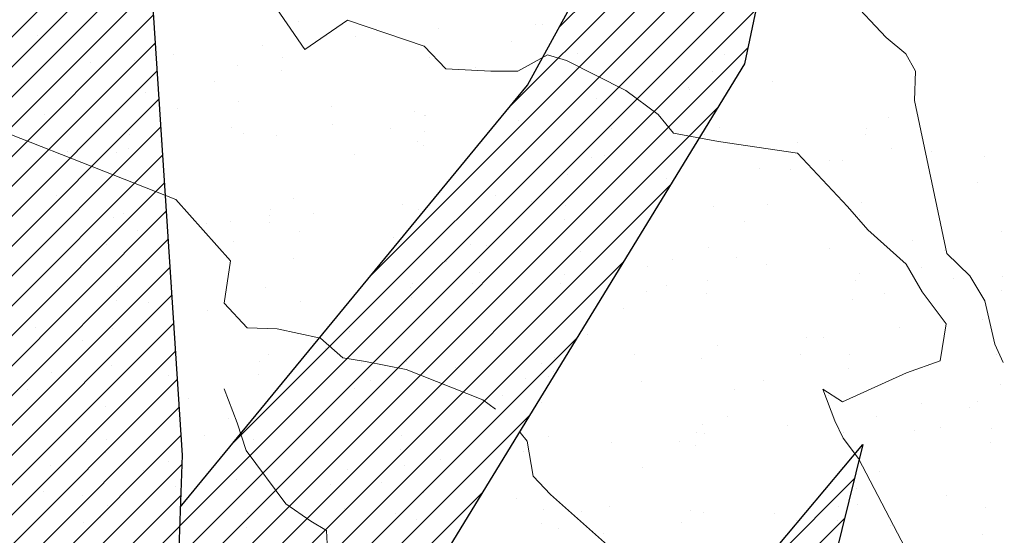
# Model space of a CAD drawing. Units: inches. Extents: x 1986 to 21484, y -1816 to 2016.
# Tile 74 of 85: x 3669.485 to 3676.656, y 1894.917 to 1898.672. Entities that reach past the tile are written whole.
import ezdxf

# ---------------------------------------------------------------- set-up
doc = ezdxf.new("R2010")
doc.units = ezdxf.units.IN
doc.layers.add('L-PLNT', color=84, linetype='Continuous', lineweight=13)
doc.layers.add('vfolhas', color=114, linetype='Continuous', lineweight=5)
doc.layers.add('vfolha2', color=110, linetype='Continuous')
doc.layers.add('vfolhas2', color=102, linetype='Continuous')
pattern_1 = [(45, (-2446.5133113, 50.986076), (-0.004419417382, 0.004419417382), [])]

# ---------------------------------------------------------------- blocks, each defined once
blk = doc.blocks.new('arbusto_PB_verde_grande')
at = {"layer": 'vfolha2'}
h = blk.add_hatch(dxfattribs=at)
h.set_pattern_fill('ANSI31', color=256, scale=0.05, style=0)
h.set_pattern_definition(pattern_1)
h.paths.add_polyline_path([(0.02944, 0.35651), (0.00028, 0.09048), (0.02625, -0.03934), (0.047, 0.06233), (0.06189, 0.09731), (0.09372, 0.26573), (0.09955, 0.43473), (0.08789, 0.61313), (0.0645, 0.72266), (0.04988, 0.6851), (0.0236, 0.51294)])
h.paths.add_polyline_path([(0.30106, 0.43789), (0.14225, 0.24871), (0.26685, 0.30022)])
h.paths.add_polyline_path([(0.37995, 0.22817), (0.23697, 0.15193), (0.18428, 0.09364), (0.11122, 0.04358), (0.02625, -0.03934), (0.28061, 0.04667), (0.36829, 0.07798), (0.46756, 0.11239), (0.61068, 0.19376), (0.71585, 0.27823), (0.55813, 0.25948)])
h.paths.add_polyline_path([(0.56101, -0.29441), (0.72752, -0.32573), (0.59024, -0.2412), (0.42962, -0.15982), (0.02625, -0.03934), (0.14922, -0.14107), (0.18838, -0.16604), (0.41501, -0.24435)])
h.paths.add_polyline_path([(-0.27429, -0.44776), (-0.30352, -0.72628), (-0.23923, -0.64175), (-0.15457, -0.45716), (0.02625, -0.03934), (-0.16328, -0.25376)])
h.paths.add_polyline_path([(-0.51963, -0.24744), (-0.67736, -0.32573), (-0.59558, -0.35072), (-0.40574, -0.32882), (-0.21007, -0.20995), (0.02625, -0.03934), (-0.14874, -0.06595), (-0.31518, -0.09101), (-0.41452, -0.15048)])
h.paths.add_polyline_path([(-0.52546, 0.25007), (-0.70947, 0.24698), (-0.51963, 0.1093), (-0.32979, 0.02167), (-0.07567, -0.0128), (-0.04234, -0.02148), (-0.35024, 0.1312)])
at = {"layer": 'vfolhas'}
h = blk.add_hatch(dxfattribs=at)
h.set_pattern_fill('ANSI31', color=256, scale=0.05, style=0)
h.set_pattern_definition(pattern_1)
h.paths.add_polyline_path([(-0.07279, 0.50669), (-0.18085, 0.65063), (-0.2334, 0.67253), (-0.20712, 0.53176), (-0.10785, 0.25007), (0.02625, -0.03934), (0.00028, 0.09048), (0.00816, 0.16241), (-0.04939, 0.29079)])
h.paths.add_polyline_path([(0.09902, 0.41929), (0.09372, 0.26573), (0.07906, 0.18814), (0.15506, 0.36901), (0.26606, 0.5505), (0.28356, 0.63504), (0.2485, 0.68819), (0.25145, 0.63504), (0.20178, 0.54426)])
h.paths.add_polyline_path([(0.12295, 0.24073), (0.047, 0.06233), (0.02625, -0.03934), (0.11122, 0.04358), (0.18428, 0.09364), (0.27478, 0.19376), (0.3215, 0.25323), (0.44129, 0.38467), (0.47634, 0.57866), (0.41789, 0.45347), (0.28939, 0.30954)])
h.paths.add_polyline_path([(0.58145, -0.03779), (0.70707, 0.01536), (0.78591, 0.04667), (0.74796, 0.06549), (0.62818, 0.08423), (0.52595, 0.09048), (0.39745, 0.04358), (0.02625, -0.03934), (0.25728, -0.03154), (0.43834, -0.0347)])
h.paths.add_polyline_path([(0.52022, -0.03647), (0.43834, -0.0347), (0.25728, -0.03154), (0.02625, -0.03934), (0.17964, -0.08515), (0.53768, -0.13167), (0.69541, -0.15357), (0.78591, -0.07852), (0.70413, -0.10042)])
h.paths.add_polyline_path([(0.27189, -0.21929), (0.14922, -0.14107), (0.02625, -0.03934), (0.15794, -0.31007), (0.29522, -0.42585), (0.41789, -0.49157), (0.56396, -0.56669), (0.5114, -0.48532), (0.39456, -0.34139)])
h.paths.add_polyline_path([(-0.05818, -0.47591), (-0.02312, -0.61984), (0.047, -0.80134), (0.08494, -0.59794), (0.07911, -0.4071), (0.03527, -0.25376), (0.02625, -0.03934), (-0.03773, -0.26001)])
h.paths.add_polyline_path([(-0.24218, 0.14054), (-0.11073, 0.06858), (0.02625, -0.03934), (-0.04235, 0.10871), (-0.21007, 0.23757), (-0.36485, 0.33145), (-0.47874, 0.40341), (-0.54303, 0.46288), (-0.49041, 0.33145), (-0.39408, 0.22192)])
at = {"layer": 'vfolha2'}
for p, q in [((0.08789, 0.61313), (0.09955, 0.43473)), ((0.14339, 0.25007), (0.30106, 0.43789)), ((0.30106, 0.43789), (0.26606, 0.29704)), ((0.09955, 0.43473), (0.09372, 0.26573))]:
    blk.add_line(p, q, dxfattribs=at)
at = {"layer": 'vfolhas2'}
for p, q in [((0.20178, 0.54426), (0.25145, 0.63504)), ((0.28356, 0.63504), (0.26606, 0.5505)), ((0.26606, 0.5505), (0.15506, 0.36901)), ((0.09902, 0.41929), (0.20178, 0.54426))]:
    blk.add_line(p, q, dxfattribs=at)
blk = doc.blocks.new('PLANT-SHRUB')
for p, q in [((2150.9894, 1887.1078), (2150.9894, 1887.1078)), ((2150.8411, 1886.9754), (2150.8411, 1886.9754)), ((2151.2728, 1886.0864), (2151.4706, 1886.7919)), ((2150.994, 1886.7216), (2150.994, 1886.7216)), ((2150.4934, 1886.6568), (2150.4934, 1886.6568)), ((2150.4197, 1886.5893), (2150.4197, 1886.5893)), ((2151.4419, 1886.6009), (2151.4419, 1886.6009)), ((2150.1488, 1886.3993), (2150.1488, 1886.3993)), ((2150.3568, 1886.3719), (2150.3568, 1886.3719)), ((2150.4298, 1886.3651), (2150.4298, 1886.3651)), ((2150.0259, 1886.2961), (2149.9795, 1886.157)), ((2150.6817, 1886.3292), (2150.6817, 1886.3292)), ((2151.5093, 1886.3263), (2151.5093, 1886.3263)), ((2151.6948, 1886.3061), (2151.6948, 1886.3061)), ((2150.0219, 1886.2248), (2150.0219, 1886.2248)), ((2150.8351, 1886.2143), (2150.8351, 1886.2143)), ((2151.2246, 1886.2577), (2151.2246, 1886.2577)), ((2151.4326, 1886.2303), (2151.4326, 1886.2303)), ((2151.6212, 1886.2385), (2151.6212, 1886.2385)), ((2149.9795, 1886.157), (2149.8169, 1885.8786)), ((2151.7575, 1886.1875), (2151.7575, 1886.1875)), ((2150.6666, 1886.107), (2150.6666, 1886.107)), ((2151.2521, 1885.9004), (2151.2728, 1886.0864)), ((2151.9112, 1886.1047), (2151.9112, 1886.1047)), ((2149.6742, 1885.9062), (2149.6742, 1885.9062)), ((2149.9227, 1885.9649), (2149.9227, 1885.9649)), ((2150.1352, 1885.8074), (2150.3524, 1885.9727)), ((2150.3524, 1885.9727), (2150.5903, 1885.8694)), ((2150.3524, 1885.9727), (2150.3524, 1885.9727)), ((2150.9689, 1885.9515), (2150.9689, 1885.9515)), ((2151.9913, 1885.9564), (2151.9913, 1885.9564)), ((2149.6005, 1885.8387), (2149.6005, 1885.8387)), ((2149.8169, 1885.8786), (2149.7705, 1885.6698)), ((2150.5903, 1885.8694), (2151.0763, 1885.7041)), ((2151.2108, 1885.7661), (2151.2521, 1885.9004)), ((2151.2234, 1885.874), (2151.2234, 1885.874)), ((2150.1042, 1885.518), (2150.1352, 1885.8074)), ((2150.1352, 1885.8074), (2150.1352, 1885.8074)), ((2151.1177, 1885.5387), (2151.2108, 1885.7661)), ((2151.2108, 1885.7661), (2151.2108, 1885.7661)), ((2151.0763, 1885.7041), (2151.1177, 1885.5387)), ((2149.7705, 1885.6698), (2149.7821, 1885.4378)), ((2149.3823, 1885.5901), (2149.3823, 1885.5901)), ((2149.8745, 1885.6023), (2149.8745, 1885.6023)), ((2150.4046, 1885.595), (2150.4046, 1885.595)), ((2150.8756, 1885.5554), (2150.8756, 1885.5554)), ((2151.1191, 1885.6001), (2151.1191, 1885.6001)), ((2151.4841, 1885.5562), (2151.4841, 1885.5562)), ((2152.3637, 1885.5978), (2152.3637, 1885.5978)), ((2150.0525, 1885.2907), (2150.1042, 1885.518)), ((2150.1042, 1885.518), (2150.1042, 1885.518)), ((2150.802, 1885.4879), (2150.802, 1885.4879)), ((2152.4248, 1885.5232), (2152.4248, 1885.5232)), ((2152.5303, 1885.5428), (2152.5303, 1885.5428)), ((2149.7821, 1885.4378), (2149.1901, 1884.4635)), ((2149.7803, 1885.413), (2149.7803, 1885.413)), ((2149.9883, 1885.3856), (2149.9883, 1885.3856)), ((2150.3132, 1885.3429), (2150.3132, 1885.3429)), ((2150.0835, 1884.9187), (2150.0525, 1885.2907)), ((2150.8561, 1885.2714), (2150.8561, 1885.2714)), ((2153.0885, 1884.7414), (2153.0373, 1885.2944)), ((2149.2677, 1885.2158), (2149.2677, 1885.2158)), ((2149.8975, 1885.1948), (2149.8975, 1885.1948)), ((2150.5124, 1885.2135), (2150.5124, 1885.2135)), ((2151.0641, 1885.244), (2151.0641, 1885.244)), ((2151.389, 1885.2012), (2151.389, 1885.2012)), ((2151.757, 1885.2113), (2151.757, 1885.2113)), ((2152.0771, 1885.2046), (2152.0771, 1885.2046)), ((2153.0016, 1885.209), (2153.0016, 1885.209)), ((2150.4042, 1885.1234), (2150.4042, 1885.1234)), ((2150.9437, 1885.1814), (2150.9437, 1885.1814)), ((2151.9319, 1885.1298), (2151.9319, 1885.1298)), ((2151.9661, 1885.1863), (2151.9661, 1885.1863)), ((2152.0034, 1885.1371), (2152.0034, 1885.1371)), ((2153.0455, 1885.1474), (2153.0455, 1885.1474)), ((2149.0992, 1885.1084), (2149.0992, 1885.1084)), ((2150.3438, 1885.1061), (2150.3438, 1885.1061)), ((2151.5885, 1885.1039), (2151.5885, 1885.1039)), ((2152.1399, 1885.1024), (2152.1399, 1885.1024)), ((2152.4649, 1885.0596), (2152.4649, 1885.0596)), ((2152.8331, 1885.1016), (2152.8331, 1885.1016)), ((2153.0077, 1884.9881), (2153.0077, 1884.9881)), ((2150.075, 1884.6914), (2150.0835, 1884.9187)), ((2153.2158, 1884.9607), (2153.2158, 1884.9607)), ((2153.2786, 1884.8538), (2153.2786, 1884.8538)), ((2149.3571, 1884.82), (2149.3571, 1884.82)), ((2150.0565, 1884.8048), (2150.0565, 1884.8048)), ((2150.3795, 1884.825), (2150.3795, 1884.825)), ((2151.4589, 1884.7861), (2151.4589, 1884.7861)), ((2151.6056, 1884.7726), (2151.6056, 1884.7726)), ((2152.5051, 1884.7727), (2152.5051, 1884.7727)), ((2153.2049, 1884.7863), (2153.2049, 1884.7863)), ((2149.9828, 1884.7373), (2149.9828, 1884.7373)), ((2150.075, 1884.1595), (2150.075, 1884.6914)), ((2153.0885, 1884.7414), (2153.0885, 1884.7414)), ((2153.0885, 1884.5571), (2153.0885, 1884.7414)), ((2149.5517, 1884.6015), (2149.5517, 1884.6015)), ((2150.7963, 1884.5992), (2150.7963, 1884.5992)), ((2152.0409, 1884.597), (2152.0409, 1884.597)), ((2152.945, 1884.3421), (2153.0885, 1884.5571)), ((2153.2856, 1884.5947), (2153.2856, 1884.5947)), ((2149.1901, 1884.4635), (2149.0392, 1884.3127)), ((2149.4118, 1884.4267), (2149.4118, 1884.4267)), ((2149.8723, 1884.4247), (2149.8723, 1884.4247)), ((2150.9185, 1884.4113), (2150.9185, 1884.4113)), ((2151.2579, 1884.454), (2151.2579, 1884.454)), ((2151.9409, 1884.4162), (2151.9409, 1884.4162)), ((2152.8071, 1884.4218), (2152.8071, 1884.4218)), ((2149.585, 1884.3728), (2149.585, 1884.3728)), ((2149.6198, 1884.3993), (2149.6198, 1884.3993)), ((2149.9447, 1884.3566), (2149.9447, 1884.3566)), ((2151.1843, 1884.3865), (2151.1843, 1884.3865)), ((2152.9398, 1884.2617), (2152.945, 1884.3421)), ((2152.945, 1884.3421), (2152.945, 1884.3421)), ((2153.0204, 1884.3773), (2153.0204, 1884.3773)), ((2149.0392, 1884.3127), (2149.0044, 1884.1735)), ((2150.4876, 1884.2851), (2150.4876, 1884.2851)), ((2150.6956, 1884.2577), (2150.6956, 1884.2577)), ((2150.1896, 1884.2127), (2150.1896, 1884.2127)), ((2151.0205, 1884.2149), (2151.0205, 1884.2149)), ((2151.4342, 1884.2104), (2151.4342, 1884.2104)), ((2152.6788, 1884.2082), (2152.6788, 1884.2082)), ((2153.9235, 1884.2059), (2153.9235, 1884.2059)), ((2154.775, 1884.1886), (2154.4569, 1883.8163)), ((2149.0044, 1884.1735), (2149.0276, 1883.9879)), ((2150.4369, 1883.7048), (2150.075, 1884.1595)), ((2151.5634, 1884.1435), (2151.5634, 1884.1435)), ((2151.7714, 1884.1161), (2151.7714, 1884.1161)), ((2150.021, 1884.1053), (2150.021, 1884.1053)), ((2150.3543, 1884.0549), (2150.3543, 1884.0549)), ((2151.2657, 1884.1031), (2151.2657, 1884.1031)), ((2152.0964, 1884.0733), (2152.0964, 1884.0733)), ((2152.4594, 1884.1032), (2152.4594, 1884.1032)), ((2152.5103, 1884.1008), (2152.5103, 1884.1008)), ((2153.7549, 1884.0985), (2153.7549, 1884.0985)), ((2154.0086, 1884.071), (2154.0086, 1884.071)), ((2149.0276, 1883.9879), (2149.0276, 1883.002)), ((2150.7865, 1884.022), (2150.7865, 1884.022)), ((2151.4338, 1884.016), (2151.4338, 1884.016)), ((2152.3857, 1884.0357), (2152.3857, 1884.0357)), ((2152.4799, 1884.0026), (2152.4799, 1884.0026)), ((2152.6392, 1884.0018), (2152.6392, 1884.0018)), ((2152.8473, 1883.9744), (2152.8473, 1883.9744)), ((2152.9758, 1883.9017), (2152.9553, 1884.0144)), ((2153.5023, 1884.0075), (2153.5023, 1884.0075)), ((2153.232, 1883.359), (2152.9758, 1883.9017)), ((2153.1722, 1883.9317), (2153.1722, 1883.9317)), ((2153.7151, 1883.8602), (2153.7151, 1883.8602)), ((2153.9231, 1883.8328), (2153.9231, 1883.8328)), ((2154.248, 1883.79), (2154.248, 1883.79)), ((2154.4569, 1883.8163), (2154.4932, 1883.6891)), ((2150.4369, 1883.7048), (2150.4369, 1883.7048)), ((2150.6334, 1883.4361), (2150.4369, 1883.7048)), ((2150.4388, 1883.7034), (2150.4388, 1883.7034)), ((2153.5872, 1883.6849), (2153.5872, 1883.6849)), ((2153.6609, 1883.7524), (2153.6609, 1883.7524)), ((2154.4932, 1883.6891), (2154.5387, 1883.4712)), ((2149.8472, 1883.6546), (2149.8472, 1883.6546)), ((2150.3651, 1883.6359), (2150.3651, 1883.6359)), ((2150.8933, 1883.6412), (2150.8933, 1883.6412)), ((2151.9157, 1883.6461), (2151.9157, 1883.6461)), ((2151.9879, 1883.6712), (2151.9879, 1883.6712)), ((2150.4735, 1883.5984), (2150.4735, 1883.5984)), ((2151.7182, 1883.5962), (2151.7182, 1883.5962)), ((2152.9628, 1883.5939), (2152.9628, 1883.5939)), ((2152.9952, 1883.6073), (2152.9952, 1883.6073)), ((2154.0414, 1883.5939), (2154.0414, 1883.5939)), ((2154.2074, 1883.5916), (2154.2074, 1883.5916)), ((2154.5387, 1883.4712), (2154.4841, 1882.9898)), ((2150.6231, 1883.2605), (2150.6334, 1883.4361)), ((2150.6334, 1883.4361), (2150.6334, 1883.4361)), ((2154.8623, 1883.4016), (2154.8623, 1883.4016)), ((2151.6402, 1883.3526), (2151.6402, 1883.3526)), ((2153.232, 1883.359), (2153.232, 1883.359)), ((2153.4062, 1883.1132), (2153.232, 1883.359)), ((2154.7887, 1883.3341), (2154.7887, 1883.3341)), ((2149.9673, 1883.2713), (2149.9673, 1883.2713)), ((2150.1191, 1883.2988), (2150.1191, 1883.2988)), ((2150.3271, 1883.2714), (2150.3271, 1883.2714)), ((2150.3291, 1883.2848), (2150.3291, 1883.2848)), ((2150.6748, 1882.9711), (2150.6231, 1883.2605)), ((2151.5666, 1883.2851), (2151.5666, 1883.2851)), ((2153.1894, 1883.3204), (2153.1894, 1883.3204)), ((2150.652, 1883.2286), (2150.652, 1883.2286)), ((2151.1114, 1883.2096), (2151.1114, 1883.2096)), ((2151.4086, 1883.2459), (2151.4086, 1883.2459)), ((2152.3561, 1883.2074), (2152.3561, 1883.2074)), ((2152.4548, 1883.2325), (2152.4548, 1883.2325)), ((2153.4772, 1883.2374), (2153.4772, 1883.2374)), ((2153.6007, 1883.2051), (2153.6007, 1883.2051)), ((2154.5566, 1883.1985), (2154.5566, 1883.1985)), ((2154.8453, 1883.2028), (2154.8453, 1883.2028)), ((2151.1949, 1883.1572), (2151.1949, 1883.1572)), ((2151.4029, 1883.1298), (2151.4029, 1883.1298)), ((2153.4062, 1883.1132), (2153.4062, 1883.1132)), ((2153.5087, 1882.9801), (2153.4062, 1883.1132)), ((2150.9429, 1883.1023), (2150.9429, 1883.1023)), ((2151.7279, 1883.087), (2151.7279, 1883.087)), ((2152.1875, 1883.1), (2152.1875, 1883.1)), ((2153.4321, 1883.0977), (2153.4321, 1883.0977)), ((2154.6768, 1883.0955), (2154.6768, 1883.0955)), ((2150.8403, 1882.5164), (2150.6748, 1882.9711)), ((2152.2707, 1883.0155), (2152.2707, 1883.0155)), ((2152.4788, 1882.9881), (2152.4788, 1882.9881)), ((2152.8417, 1883.0018), (2152.8417, 1883.0018)), ((2153.5292, 1882.765), (2153.5087, 1882.9801)), ((2154.3909, 1882.9696), (2154.3909, 1882.9696)), ((2154.4841, 1882.9898), (2154.3932, 1882.7991)), ((2151.1687, 1882.9206), (2151.1687, 1882.9206)), ((2152.768, 1882.9343), (2152.768, 1882.9343)), ((2152.8037, 1882.9454), (2152.8037, 1882.9454)), ((2150.8682, 1882.8711), (2150.8682, 1882.8711)), ((2151.8905, 1882.876), (2151.8905, 1882.876)), ((2152.97, 1882.8372), (2152.97, 1882.8372)), ((2153.3466, 1882.8739), (2153.3466, 1882.8739)), ((2153.5546, 1882.8465), (2153.5546, 1882.8465)), ((2154.0162, 1882.8238), (2154.0162, 1882.8238)), ((2155.0386, 1882.8287), (2155.0386, 1882.8287)), ((2153.7137, 1882.4988), (2153.5292, 1882.765)), ((2153.8795, 1882.8037), (2153.8795, 1882.8037)), ((2154.3932, 1882.7991), (2154.2933, 1882.5539)), ((2154.4224, 1882.7323), (2154.4224, 1882.7323)), ((2154.6304, 1882.7049), (2154.6304, 1882.7049)), ((2154.0431, 1882.651), (2154.0431, 1882.651)), ((2154.9553, 1882.6621), (2154.9553, 1882.6621)), ((2155.5923, 1882.6188), (2155.5923, 1882.6188)), ((2150.821, 1882.6019), (2150.821, 1882.6019)), ((2151.3954, 1882.5953), (2151.3954, 1882.5953)), ((2152.3702, 1882.5698), (2152.3702, 1882.5698)), ((2152.64, 1882.5931), (2152.64, 1882.5931)), ((2153.8846, 1882.5908), (2153.8846, 1882.5908)), ((2153.9695, 1882.5835), (2153.9695, 1882.5835)), ((2155.1293, 1882.5886), (2155.1293, 1882.5886)), ((2155.4982, 1882.5906), (2155.4982, 1882.5906)), ((2155.7062, 1882.5632), (2155.7062, 1882.5632)), ((2150.7474, 1882.5344), (2150.7474, 1882.5344)), ((2150.9127, 1882.3924), (2150.8403, 1882.5164)), ((2151.3834, 1882.4758), (2151.3834, 1882.4758)), ((2153.452, 1882.4673), (2153.452, 1882.4673)), ((2153.8674, 1882.3451), (2153.7137, 1882.4988)), ((2151.1505, 1882.3304), (2150.9127, 1882.3924)), ((2152.4296, 1882.4624), (2152.4296, 1882.4624)), ((2154.5314, 1882.4284), (2154.5314, 1882.4284)), ((2155.5776, 1882.4151), (2155.5776, 1882.4151)), ((2151.2953, 1882.1961), (2151.1505, 1882.3304)), ((2153.8674, 1882.0994), (2153.8674, 1882.3451)), ((2152.0225, 1882.2512), (2152.0225, 1882.2512)), ((2155.2446, 1882.3002), (2155.2446, 1882.3002)), ((2150.7886, 1882.2088), (2150.7886, 1882.2088)), ((2151.5228, 1881.9584), (2151.2953, 1882.1961)), ((2151.9488, 1882.1836), (2151.9488, 1882.1836)), ((2152.0333, 1882.2065), (2152.0333, 1882.2065)), ((2153.2779, 1882.2043), (2153.2779, 1882.2043)), ((2153.5717, 1882.219), (2153.5717, 1882.219)), ((2154.5225, 1882.202), (2154.5225, 1882.202)), ((2155.1709, 1882.2327), (2155.1709, 1882.2327)), ((2155.7672, 1882.1998), (2155.7672, 1882.1998)), ((2150.8264, 1882.1709), (2150.8264, 1882.1709)), ((2151.0345, 1882.1435), (2151.0345, 1882.1435)), ((2151.8654, 1882.1059), (2151.8654, 1882.1059)), ((2151.3594, 1882.1007), (2151.3594, 1882.1007)), ((2151.8647, 1882.0992), (2151.8647, 1882.0992)), ((2152.9448, 1882.0671), (2152.9448, 1882.0671)), ((2153.1094, 1882.0969), (2153.1094, 1882.0969)), ((2153.6229, 1881.9049), (2153.8674, 1882.0994)), ((2153.991, 1882.0537), (2153.991, 1882.0537)), ((2154.354, 1882.0946), (2154.354, 1882.0946)), ((2155.0134, 1882.0586), (2155.0134, 1882.0586)), ((2155.5986, 1882.0924), (2155.5986, 1882.0924)), ((2151.9022, 1882.0292), (2151.9022, 1882.0292)), ((2152.1103, 1882.0018), (2152.1103, 1882.0018)), ((2151.5228, 1881.7311), (2151.5228, 1881.9584)), ((2152.4352, 1881.9591), (2152.4352, 1881.9591)), ((2153.224, 1881.9004), (2153.224, 1881.9004)), ((2153.6083, 1881.3076), (2153.6229, 1881.9049)), ((2153.6229, 1881.9049), (2153.6229, 1881.9049)), ((2151.551, 1881.8191), (2151.551, 1881.8191)), ((2152.9781, 1881.8876), (2152.9781, 1881.8876)), ((2153.1503, 1881.8329), (2153.1503, 1881.8329)), ((2153.1861, 1881.8602), (2153.1861, 1881.8602)), ((2154.7731, 1881.8682), (2154.7731, 1881.8682)), ((2153.511, 1881.8174), (2153.511, 1881.8174)), ((2151.3582, 1881.7057), (2151.3582, 1881.7057)), ((2151.8029, 1881.2105), (2151.5228, 1881.7311)), ((2152.4044, 1881.6923), (2152.4044, 1881.6923)), ((2153.4268, 1881.6972), (2153.4268, 1881.6972)), ((2154.0539, 1881.746), (2154.0539, 1881.746)), ((2154.2619, 1881.7186), (2154.2619, 1881.7186)), ((2154.5868, 1881.6758), (2154.5868, 1881.6758)), ((2154.5063, 1881.6583), (2154.5063, 1881.6583)), ((2155.1297, 1881.6043), (2155.1297, 1881.6043)), ((2152.3172, 1881.5923), (2152.3172, 1881.5923)), ((2153.5619, 1881.59), (2153.5619, 1881.59)), ((2154.4254, 1881.5496), (2154.4254, 1881.5496)), ((2154.8065, 1881.5877), (2154.8065, 1881.5877)), ((2155.3377, 1881.5769), (2155.3377, 1881.5769)), ((2152.7525, 1881.4683), (2152.7525, 1881.4683)), ((2154.3518, 1881.4821), (2154.3518, 1881.4821)), ((2151.8402, 1881.3359), (2151.8402, 1881.3359)), ((2152.9197, 1881.297), (2152.9197, 1881.297)), ((2153.6083, 1881.3076), (2153.6083, 1881.3076)), ((2154.164, 1880.1332), (2153.6083, 1881.3076)), ((2153.9658, 1881.2836), (2153.9658, 1881.2836)), ((2154.9882, 1881.2885), (2154.9882, 1881.2885)), ((2152.174, 1881.1542), (2151.8029, 1881.2105)), ((2152.9551, 1881.2035), (2152.9551, 1881.2035)), ((2154.1997, 1881.2012), (2154.1997, 1881.2012)), ((2152.0694, 1880.4639), (2152.174, 1881.1542)), ((2152.4048, 1881.1497), (2152.4048, 1881.1497)), ((2153.954, 1881.1176), (2153.954, 1881.1176)), ((2152.3311, 1881.0822), (2152.3311, 1881.0822)), ((2152.7866, 1881.0961), (2152.7866, 1881.0961)), ((2154.0312, 1881.0938), (2154.0312, 1881.0938)), ((2152.0667, 1880.9728), (2152.0667, 1880.9728)), ((2152.3792, 1880.9222), (2152.3792, 1880.9222)), ((2152.6096, 1880.9013), (2152.6096, 1880.9013)), ((2153.4016, 1880.9271), (2153.4016, 1880.9271)), ((2154.4811, 1880.8882), (2154.4811, 1880.8882)), ((2152.8176, 1880.8739), (2152.8176, 1880.8739)), ((2153.1425, 1880.8311), (2153.1425, 1880.8311)), ((2153.6062, 1880.799), (2153.6062, 1880.799)), ((2153.6854, 1880.7597), (2153.6854, 1880.7597)), ((2153.5326, 1880.7314), (2153.5326, 1880.7314)), ((2153.8934, 1880.7323), (2153.8934, 1880.7323)), ((2154.2184, 1880.6895), (2154.2184, 1880.6895)), ((2153.2391, 1880.5892), (2153.2391, 1880.5892)), ((2154.4837, 1880.5869), (2154.4837, 1880.5869)), ((2152.8945, 1880.5269), (2152.8945, 1880.5269)), ((2153.9407, 1880.5135), (2153.9407, 1880.5135)), ((2153.1348, 1880.3669), (2153.1348, 1880.3669)), ((2153.877, 1880.2004), (2153.877, 1880.2004)), ((2153.3764, 1880.157), (2153.3764, 1880.157)), ((2153.7084, 1880.093), (2153.7084, 1880.093)), ((2153.5249, 1879.746), (2153.5249, 1879.746))]:
    blk.add_line(p, q)

msp = doc.modelspace()

# ---------------------------------------------------------------- block references
at = {"layer": 'L-PLNT', "rotation": 223.1883365522388}
msp.add_blockref('PLANT-SHRUB', (3953.27, 4742.9646), dxfattribs=at)
at = {"layer": 'L-PLNT', "xscale": 24.60366729364114, "yscale": 24.60366729364114, "zscale": 24.60366729364114}
msp.add_blockref('arbusto_PB_verde_grande', (3668.2184, 1884.8051), dxfattribs=at)

doc.saveas('drawing.dxf')
